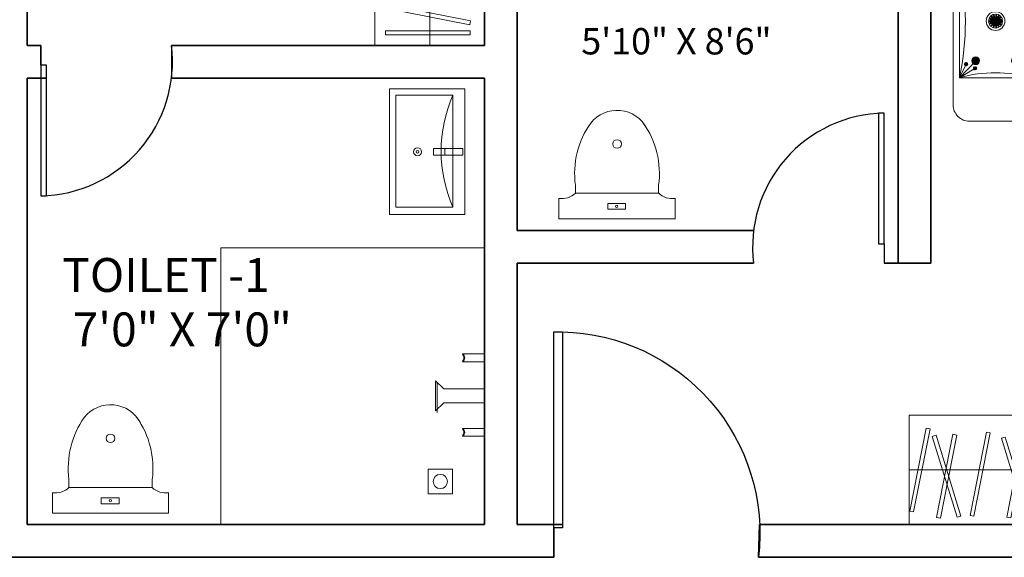
# Model space of a CAD drawing. Units: inches. Extents: x -61 to 1599, y -1316 to 257.
# Tile 171 of 204: x 1214 to 1395, y -783 to -684. Entities that reach past the tile are written whole.
import ezdxf

# ---------------------------------------------------------------- set-up
doc = ezdxf.new("R2010")
doc.units = ezdxf.units.IN
doc.header["$MEASUREMENT"] = 0
doc.linetypes.add('ACAD_ISO02W100', pattern=[15, 12, -3])
for name, color, linetype, lineweight in [('A-AREA-IDEN', 1, 'Continuous', 18), ('A-FLOR-CASE', 8, 'Continuous', 18), ('A-FLOR-FIXT', 8, 'Continuous', 18), ('A-WALL-JAMB', 4, 'ACAD_ISO02W100', 25), ('DOORS', 2, 'Continuous', 25), ('FURNITURE', 83, 'Continuous', 18), ('WALLS', 4, 'Continuous', 35)]:
    doc.layers.add(name, color=color, linetype=linetype, lineweight=lineweight)
doc.layers.add('LT', color=8, linetype='Continuous')
doc.styles.get("Standard").update_dxf_attribs({"font": 'arial.ttf'})

# ---------------------------------------------------------------- blocks, each defined once
blk = doc.blocks.new('DOOR-SWING-24')
blk.add_line((0, 0), (0, 3.6))
blk.add_lwpolyline([(0, 0), (0, -24), (1.05, -24), (1.05, 0)], close=True)
blk.add_arc((-0.44, 0.62), 24.62, 271.0259, 6.9559)
blk = doc.blocks.new('DOOR-SWING-36')
blk.add_line((0, 0), (0, -5.4))
blk.add_lwpolyline([(0, 0), (0, 36), (-1.57, 36), (-1.57, 0)], close=True)
blk.add_arc((-0.74, -1.08), 37.09, 91.2913, 186.6905)
blk = doc.blocks.new('WC-FLOOR-MOUNT')
for p, q in [((3.02, 4.69), (3.02, 6.17)), ((18.31, 4.69), (18.31, 6.17)), ((0, 0), (0, 3.75)), ((3.02, 4.69), (18.31, 4.69)), ((21.33, 0), (21.33, 3.75)), ((0, 0), (21.33, 0))]:
    blk.add_line(p, q)
blk.add_lwpolyline([(12.24, 1.73), (8.96, 1.73), (8.96, 2.81), (12.24, 2.81)], close=True)
for centre, radius in [((10.67, 13.73), 0.792), ((10.6, 2.27), 0.208)]:
    blk.add_circle(centre, radius)
for centre, radius, start, end in [((10.67, 13.73), 6.18, 27.6844, 141.4697), ((19.05, 8.26), 16.17, 144.824, 187.4232), ((2.28, 8.26), 16.17, 352.5768, 35.176), ((0.56, 7.25), 3.55, 260.8586, 313.6993), ((20.77, 7.25), 3.55, 226.3007, 279.1414)]:
    blk.add_arc(centre, radius, start, end)
blk = doc.blocks.new('LAVATORY-WALL')
blk.add_line((10.19, 12.11), (10.19, 10.88))
for points in [[(13.87, 0), (0, 0), (0, 23.07), (13.87, 23.07)], [(13.87, 0), (0, 0), (0, 23.07), (13.87, 23.07)], [(1.2, 1.34), (1.2, 21.88), (11.67, 21.88), (11.67, 1.34)], [(8.09, 10.88), (8.09, 12.11), (13.47, 12.11), (13.47, 10.88)]]:
    blk.add_lwpolyline(points, close=True)
for radius in [0.74, 0.233]:
    blk.add_circle((5.16, 11.5), radius)
blk.add_arc((34.73, 11.61), 25.25, 155.9939, 204.0061)
blk = doc.blocks.new('SHOWER-FITTINGS')
for p, q in [((10.35, 25.72), (6.31, 25.72)), ((10.35, 24.3), (6.31, 24.3)), ((10.35, 23), (10.35, 23)), ((2.92, 19.29), (1.4, 20.76)), ((1.4, 15.27), (1.4, 20.76)), ((1.69, 14.98), (1.69, 20.48)), ((10.35, 19.29), (2.92, 19.29)), ((2.92, 16.74), (1.4, 15.27)), ((10.35, 16.74), (2.92, 16.74)), ((10.35, 12.03), (6.31, 12.03)), ((10.35, 10.61), (6.31, 10.61))]:
    blk.add_line(p, q)
blk.add_lwpolyline([(4.52, 0), (0, 0), (0, 4.57), (4.52, 4.57)], close=True)
blk.add_circle((2.26, 2.29), 1.31)
for points in [[(6.31, 24.3), (6.45, 24.53), (6.75, 25), (6.46, 25.48), (6.31, 25.72)], [(6.45, 24.3), (6.59, 24.53), (6.88, 25), (6.59, 25.48), (6.45, 25.72)], [(6.31, 10.61), (6.45, 10.84), (6.75, 11.31), (6.46, 11.78), (6.31, 12.03)], [(6.45, 10.61), (6.59, 10.84), (6.88, 11.31), (6.59, 11.78), (6.45, 12.03)]]:
    blk.add_open_spline(points, degree=3, knots=[0, 0, 0, 0, 0.7501, 1.532449, 1.532449, 1.532449, 1.532449])
blk = doc.blocks.new('WARDROBE-HANGING')
blk.add_line((10.05, 0), (10.05, 68))
for points in [[(20.09, 0), (0, 0), (0, 68), (20.09, 68)], [(2.48, 67.85), (17.75, 64.85), (17.61, 64.14), (2.34, 67.15)], [(1.35, 59.16), (16.22, 63.73), (16.43, 63.04), (1.56, 58.47)], [(1.32, 62.96), (16.59, 59.95), (16.45, 59.25), (1.19, 62.25)], [(1.71, 56.78), (16.98, 53.78), (16.84, 53.07), (1.57, 56.08)], [(1, 46.47), (15.87, 51.04), (16.08, 50.35), (1.21, 45.78)], [(1.39, 50.01), (16.66, 47.01), (16.52, 46.3), (1.26, 49.31)], [(1.36, 44.09), (16.63, 41.09), (16.49, 40.38), (1.23, 43.38)], [(1.26, 37.2), (16.53, 34.2), (16.39, 33.49), (1.12, 36.5)], [(1.28, 33.41), (16.16, 37.98), (16.37, 37.29), (1.49, 32.72)], [(1.65, 31.03), (16.92, 28.03), (16.78, 27.32), (1.51, 30.32)], [(1.28, 21.3), (16.15, 25.87), (16.36, 25.18), (1.49, 20.61)], [(1.26, 25.09), (16.53, 22.09), (16.39, 21.38), (1.12, 24.39)], [(1.65, 18.92), (16.91, 15.92), (16.78, 15.21), (1.51, 18.21)], [(1.91, 13.69), (17.17, 10.68), (17.04, 9.98), (1.77, 12.98)], [(1.93, 9.89), (16.8, 14.46), (17.01, 13.77), (2.14, 9.2)], [(2.29, 7.51), (17.56, 4.51), (17.42, 3.8), (2.16, 6.81)], [(17.49, 1.96), (1.93, 1.96), (1.93, 2.68), (17.49, 2.68)]]:
    blk.add_lwpolyline(points, close=True)
blk = doc.blocks.new('*U100')
at = {"layer": 'LT'}
blk.add_line((0, 0.15), (0, -0.15), dxfattribs=at)
for centre, start, end in [((0.44, 0), 160.9983, 199.0017), ((-0.44, 0), 340.9983, 19.0017)]:
    blk.add_arc(centre, 0.468, start, end, dxfattribs=at)
blk = doc.blocks.new('*U101')
at = {"layer": 'LT', "transparency": 16777216}
for p, rotation in [((-57.96, -16.31), 72), ((-57.93, -16.26), 48.00000000000001), ((-57.87, -16.22), 24), ((-57.75, -16.22), 336), ((-57.7, -16.26), 312), ((-57.67, -16.31), 288), ((-57.96, -16.37), 96), ((-57.94, -16.43), 120), ((-57.9, -16.48), 144), ((-57.84, -16.51), 168.0000000000001), ((-57.78, -16.51), 192), ((-57.72, -16.48), 216), ((-57.68, -16.43), 240), ((-57.66, -16.37), 264)]:
    blk.add_blockref('*U100', p, dxfattribs=dict(at, rotation=rotation))
blk.add_blockref('*U100', (-57.81, -16.21), dxfattribs=at)
blk = doc.blocks.new('*U104')
at = {"layer": 'LT'}
blk.add_line((0, 0.15), (0, -0.15), dxfattribs=at)
for centre, start, end in [((0.44, 0), 160.9983, 199.0017), ((-0.44, 0), 340.9983, 19.0017)]:
    blk.add_arc(centre, 0.468, start, end, dxfattribs=at)
blk = doc.blocks.new('*U105')
at = {"layer": 'LT', "transparency": 16777216}
for p, rotation in [((-57.96, -16.31), 72), ((-57.93, -16.26), 48.00000000000001), ((-57.87, -16.22), 24), ((-57.75, -16.22), 336), ((-57.7, -16.26), 312), ((-57.67, -16.31), 288), ((-57.96, -16.37), 96), ((-57.94, -16.43), 120), ((-57.9, -16.48), 144), ((-57.84, -16.51), 168.0000000000001), ((-57.78, -16.51), 192), ((-57.72, -16.48), 216), ((-57.68, -16.43), 240), ((-57.66, -16.37), 264)]:
    blk.add_blockref('*U104', p, dxfattribs=dict(at, rotation=rotation))
blk.add_blockref('*U104', (-57.81, -16.21), dxfattribs=at)
blk = doc.blocks.new('*U71')
at = {"layer": 'LT'}
blk.add_line((0, 0.15), (0, -0.15), dxfattribs=at)
for centre, start, end in [((0.44, 0), 160.9983, 199.0017), ((-0.44, 0), 340.9983, 19.0017)]:
    blk.add_arc(centre, 0.468, start, end, dxfattribs=at)
blk = doc.blocks.new('*U58')
at = {"layer": 'LT', "transparency": 16777216}
for p, rotation in [((-57.96, -16.31), 72), ((-57.93, -16.26), 48.00000000000001), ((-57.87, -16.22), 24), ((-57.75, -16.22), 336), ((-57.7, -16.26), 312), ((-57.67, -16.31), 288), ((-57.96, -16.37), 96), ((-57.94, -16.43), 120), ((-57.9, -16.48), 144), ((-57.84, -16.51), 168.0000000000001), ((-57.78, -16.51), 192), ((-57.72, -16.48), 216), ((-57.68, -16.43), 240), ((-57.66, -16.37), 264)]:
    blk.add_blockref('*U71', p, dxfattribs=dict(at, rotation=rotation))
blk.add_blockref('*U71', (-57.81, -16.21), dxfattribs=at)
blk = doc.blocks.new('*U61')
at = {"layer": 'LT'}
blk.add_line((0, 0.15), (0, -0.15), dxfattribs=at)
for centre, start, end in [((0.44, 0), 160.9983, 199.0017), ((-0.44, 0), 340.9983, 19.0017)]:
    blk.add_arc(centre, 0.468, start, end, dxfattribs=at)
blk = doc.blocks.new('*U62')
at = {"layer": 'LT', "transparency": 16777216}
for p, rotation in [((-57.96, -16.31), 72), ((-57.93, -16.26), 48.00000000000001), ((-57.87, -16.22), 24), ((-57.75, -16.22), 336), ((-57.7, -16.26), 312), ((-57.67, -16.31), 288), ((-57.96, -16.37), 96), ((-57.94, -16.43), 120), ((-57.9, -16.48), 144), ((-57.84, -16.51), 168.0000000000001), ((-57.78, -16.51), 192), ((-57.72, -16.48), 216), ((-57.68, -16.43), 240), ((-57.66, -16.37), 264)]:
    blk.add_blockref('*U61', p, dxfattribs=dict(at, rotation=rotation))
blk.add_blockref('*U61', (-57.81, -16.21), dxfattribs=at)
blk = doc.blocks.new('*U94')
at = {"layer": 'LT'}
blk.add_line((0, 0.36), (0, -0.36), dxfattribs=at)
for centre, start, end in [((1.04, 0), 160.9983, 199.0017), ((-1.04, 0), 340.9983, 19.0017)]:
    blk.add_arc(centre, 1.1, start, end, dxfattribs=at)
blk = doc.blocks.new('*U95')
at = {"layer": 'LT', "transparency": 16777216}
for p, rotation in [((-136.23, -38.23), 48.00000000000001), ((-136.11, -38.14), 23.99999999999999), ((-135.82, -38.14), 336.0000000000001), ((-135.69, -38.23), 312), ((-136.32, -38.51), 96), ((-136.3, -38.36), 72), ((-136.27, -38.65), 120), ((-136.17, -38.76), 144), ((-136.04, -38.82), 168.0000000000001), ((-135.89, -38.82), 191.9999999999999), ((-135.75, -38.76), 216), ((-135.65, -38.65), 240), ((-135.62, -38.36), 288.0000000000001), ((-135.6, -38.51), 264)]:
    blk.add_blockref('*U94', p, dxfattribs=dict(at, rotation=rotation))
blk.add_blockref('*U94', (-135.96, -38.11), dxfattribs=at)
blk = doc.blocks.new('*U57')
at = {"layer": 'LT'}
blk.add_line((0, 0.36), (0, -0.36), dxfattribs=at)
for centre, start, end in [((1.04, 0), 160.9983, 199.0017), ((-1.04, 0), 340.9983, 19.0017)]:
    blk.add_arc(centre, 1.1, start, end, dxfattribs=at)
blk = doc.blocks.new('*U99')
at = {"layer": 'LT', "transparency": 16777216}
for p, rotation in [((-136.23, -38.23), 48.00000000000001), ((-136.11, -38.14), 23.99999999999999), ((-135.82, -38.14), 336.0000000000001), ((-135.69, -38.23), 312), ((-136.32, -38.51), 96), ((-136.3, -38.36), 72), ((-136.27, -38.65), 120), ((-136.17, -38.76), 144), ((-136.04, -38.82), 168.0000000000001), ((-135.89, -38.82), 191.9999999999999), ((-135.75, -38.76), 216), ((-135.65, -38.65), 240), ((-135.62, -38.36), 288.0000000000001), ((-135.6, -38.51), 264)]:
    blk.add_blockref('*U57', p, dxfattribs=dict(at, rotation=rotation))
blk.add_blockref('*U57', (-135.96, -38.11), dxfattribs=at)
blk = doc.blocks.new('*U80')
at = {"layer": 'LT'}
blk.add_line((0, 0.36), (0, -0.36), dxfattribs=at)
for centre, start, end in [((1.04, 0), 160.9983, 199.0017), ((-1.04, 0), 340.9983, 19.0017)]:
    blk.add_arc(centre, 1.1, start, end, dxfattribs=at)
blk = doc.blocks.new('*U96')
at = {"layer": 'LT', "transparency": 16777216}
for p, rotation in [((-136.23, -38.23), 48.00000000000001), ((-136.11, -38.14), 23.99999999999999), ((-135.82, -38.14), 336.0000000000001), ((-135.69, -38.23), 312), ((-136.32, -38.51), 96), ((-136.3, -38.36), 72), ((-136.27, -38.65), 120), ((-136.17, -38.76), 144), ((-136.04, -38.82), 168.0000000000001), ((-135.89, -38.82), 191.9999999999999), ((-135.75, -38.76), 216), ((-135.65, -38.65), 240), ((-135.62, -38.36), 288.0000000000001), ((-135.6, -38.51), 264)]:
    blk.add_blockref('*U80', p, dxfattribs=dict(at, rotation=rotation))
blk.add_blockref('*U80', (-135.96, -38.11), dxfattribs=at)
blk = doc.blocks.new('*U69')
at = {"layer": 'LT'}
blk.add_line((0, 0.36), (0, -0.36), dxfattribs=at)
for centre, start, end in [((1.04, 0), 160.9983, 199.0017), ((-1.04, 0), 340.9983, 19.0017)]:
    blk.add_arc(centre, 1.1, start, end, dxfattribs=at)
blk = doc.blocks.new('*U70')
at = {"layer": 'LT', "transparency": 16777216}
for p, rotation in [((-136.23, -38.23), 48.00000000000001), ((-136.11, -38.14), 23.99999999999999), ((-135.82, -38.14), 336.0000000000001), ((-135.69, -38.23), 312), ((-136.32, -38.51), 96), ((-136.3, -38.36), 72), ((-136.27, -38.65), 120), ((-136.17, -38.76), 144), ((-136.04, -38.82), 168.0000000000001), ((-135.89, -38.82), 191.9999999999999), ((-135.75, -38.76), 216), ((-135.65, -38.65), 240), ((-135.62, -38.36), 288.0000000000001), ((-135.6, -38.51), 264)]:
    blk.add_blockref('*U69', p, dxfattribs=dict(at, rotation=rotation))
blk.add_blockref('*U69', (-135.96, -38.11), dxfattribs=at)
blk = doc.blocks.new('*U102')
at = {"layer": 'LT'}
blk.add_line((0, 0.15), (0, -0.15), dxfattribs=at)
for centre, start, end in [((0.44, 0), 160.9983, 199.0017), ((-0.44, 0), 340.9983, 19.0017)]:
    blk.add_arc(centre, 0.468, start, end, dxfattribs=at)
blk = doc.blocks.new('*U103')
at = {"layer": 'LT', "transparency": 16777216}
for p, rotation in [((-57.96, -16.31), 72), ((-57.93, -16.26), 48.00000000000001), ((-57.87, -16.22), 24), ((-57.75, -16.22), 336), ((-57.7, -16.26), 312), ((-57.67, -16.31), 288), ((-57.96, -16.37), 96), ((-57.94, -16.43), 120), ((-57.9, -16.48), 144), ((-57.84, -16.51), 168.0000000000001), ((-57.78, -16.51), 192), ((-57.72, -16.48), 216), ((-57.68, -16.43), 240), ((-57.66, -16.37), 264)]:
    blk.add_blockref('*U102', p, dxfattribs=dict(at, rotation=rotation))
blk.add_blockref('*U102', (-57.81, -16.21), dxfattribs=at)
blk = doc.blocks.new('*U55')
at = {"layer": 'LT'}
blk.add_line((0, 0.15), (0, -0.15), dxfattribs=at)
for centre, start, end in [((0.44, 0), 160.9983, 199.0017), ((-0.44, 0), 340.9983, 19.0017)]:
    blk.add_arc(centre, 0.468, start, end, dxfattribs=at)
blk = doc.blocks.new('*U56')
at = {"layer": 'LT', "transparency": 16777216}
for p, rotation in [((-57.96, -16.31), 72), ((-57.93, -16.26), 48.00000000000001), ((-57.87, -16.22), 24), ((-57.75, -16.22), 336), ((-57.7, -16.26), 312), ((-57.67, -16.31), 288), ((-57.96, -16.37), 96), ((-57.94, -16.43), 120), ((-57.9, -16.48), 144), ((-57.84, -16.51), 168.0000000000001), ((-57.78, -16.51), 192), ((-57.72, -16.48), 216), ((-57.68, -16.43), 240), ((-57.66, -16.37), 264)]:
    blk.add_blockref('*U55', p, dxfattribs=dict(at, rotation=rotation))
blk.add_blockref('*U55', (-57.81, -16.21), dxfattribs=at)
blk = doc.blocks.new('*U59')
at = {"layer": 'LT'}
blk.add_line((0, 0.15), (0, -0.15), dxfattribs=at)
for centre, start, end in [((0.44, 0), 160.9983, 199.0017), ((-0.44, 0), 340.9983, 19.0017)]:
    blk.add_arc(centre, 0.468, start, end, dxfattribs=at)
blk = doc.blocks.new('*U60')
at = {"layer": 'LT', "transparency": 16777216}
for p, rotation in [((-57.96, -16.31), 72), ((-57.93, -16.26), 48.00000000000001), ((-57.87, -16.22), 24), ((-57.75, -16.22), 336), ((-57.7, -16.26), 312), ((-57.67, -16.31), 288), ((-57.96, -16.37), 96), ((-57.94, -16.43), 120), ((-57.9, -16.48), 144), ((-57.84, -16.51), 168.0000000000001), ((-57.78, -16.51), 192), ((-57.72, -16.48), 216), ((-57.68, -16.43), 240), ((-57.66, -16.37), 264)]:
    blk.add_blockref('*U59', p, dxfattribs=dict(at, rotation=rotation))
blk.add_blockref('*U59', (-57.81, -16.21), dxfattribs=at)
blk = doc.blocks.new('*U67')
at = {"layer": 'LT'}
blk.add_line((0, 0.15), (0, -0.15), dxfattribs=at)
for centre, start, end in [((0.44, 0), 160.9983, 199.0017), ((-0.44, 0), 340.9983, 19.0017)]:
    blk.add_arc(centre, 0.468, start, end, dxfattribs=at)
blk = doc.blocks.new('*U68')
at = {"layer": 'LT', "transparency": 16777216}
for p, rotation in [((-57.96, -16.31), 72), ((-57.93, -16.26), 48.00000000000001), ((-57.87, -16.22), 24), ((-57.75, -16.22), 336), ((-57.7, -16.26), 312), ((-57.67, -16.31), 288), ((-57.96, -16.37), 96), ((-57.94, -16.43), 120), ((-57.9, -16.48), 144), ((-57.84, -16.51), 168.0000000000001), ((-57.78, -16.51), 192), ((-57.72, -16.48), 216), ((-57.68, -16.43), 240), ((-57.66, -16.37), 264)]:
    blk.add_blockref('*U67', p, dxfattribs=dict(at, rotation=rotation))
blk.add_blockref('*U67', (-57.81, -16.21), dxfattribs=at)
blk = doc.blocks.new('*U106')
at = {"layer": 'LT'}
blk.add_line((0, 0.64), (0, -0.64), dxfattribs=at)
for centre, start, end in [((1.87, 0), 160.9983, 199.0017), ((-1.87, 0), 340.9983, 19.0017)]:
    blk.add_arc(centre, 1.97, start, end, dxfattribs=at)
blk = doc.blocks.new('*U93')
at = {"layer": 'LT', "transparency": 16777216}
for p, rotation in [((-244.33, -68.76), 72), ((-244.2, -68.53), 48.00000000000001), ((-243.98, -68.38), 23.99999999999999), ((-243.46, -68.38), 336.0000000000001), ((-243.25, -68.53), 312), ((-243.11, -68.76), 288), ((-244.36, -69.03), 96), ((-244.28, -69.28), 120), ((-244.1, -69.48), 144), ((-243.86, -69.59), 168), ((-243.59, -69.59), 192), ((-243.34, -69.48), 216), ((-243.17, -69.28), 240), ((-243.08, -69.03), 264)]:
    blk.add_blockref('*U106', p, dxfattribs=dict(at, rotation=rotation))
blk.add_blockref('*U106', (-243.72, -68.32), dxfattribs=at)
blk = doc.blocks.new('*U63')
at = {"layer": 'LT'}
blk.add_line((0, 0.64), (0, -0.64), dxfattribs=at)
for centre, start, end in [((1.87, 0), 160.9983, 199.0017), ((-1.87, 0), 340.9983, 19.0017)]:
    blk.add_arc(centre, 1.97, start, end, dxfattribs=at)
blk = doc.blocks.new('*U64')
at = {"layer": 'LT', "transparency": 16777216}
for p, rotation in [((-244.33, -68.76), 72), ((-244.2, -68.53), 48.00000000000001), ((-243.98, -68.38), 23.99999999999999), ((-243.46, -68.38), 336.0000000000001), ((-243.25, -68.53), 312), ((-243.11, -68.76), 288), ((-244.36, -69.03), 96), ((-244.28, -69.28), 120), ((-244.1, -69.48), 144), ((-243.86, -69.59), 168), ((-243.59, -69.59), 192), ((-243.34, -69.48), 216), ((-243.17, -69.28), 240), ((-243.08, -69.03), 264)]:
    blk.add_blockref('*U63', p, dxfattribs=dict(at, rotation=rotation))
blk.add_blockref('*U63', (-243.72, -68.32), dxfattribs=at)
blk = doc.blocks.new('*U83')
at = {"layer": 'LT'}
blk.add_line((0, 0.36), (0, -0.36), dxfattribs=at)
for centre, start, end in [((1.04, 0), 160.9983, 199.0017), ((-1.04, 0), 340.9983, 19.0017)]:
    blk.add_arc(centre, 1.1, start, end, dxfattribs=at)
blk = doc.blocks.new('*U84')
at = {"layer": 'LT', "transparency": 16777216}
for p, rotation in [((-136.23, -38.23), 48.00000000000001), ((-136.11, -38.14), 23.99999999999999), ((-135.82, -38.14), 336.0000000000001), ((-135.69, -38.23), 312), ((-136.32, -38.51), 96), ((-136.3, -38.36), 72), ((-136.27, -38.65), 120), ((-136.17, -38.76), 144), ((-136.04, -38.82), 168.0000000000001), ((-135.89, -38.82), 191.9999999999999), ((-135.75, -38.76), 216), ((-135.65, -38.65), 240), ((-135.62, -38.36), 288.0000000000001), ((-135.6, -38.51), 264)]:
    blk.add_blockref('*U83', p, dxfattribs=dict(at, rotation=rotation))
blk.add_blockref('*U83', (-135.96, -38.11), dxfattribs=at)
blk = doc.blocks.new('*U74')
at = {"layer": 'LT'}
blk.add_line((0, 0.36), (0, -0.36), dxfattribs=at)
for centre, start, end in [((1.04, 0), 160.9983, 199.0017), ((-1.04, 0), 340.9983, 19.0017)]:
    blk.add_arc(centre, 1.1, start, end, dxfattribs=at)
blk = doc.blocks.new('*U75')
at = {"layer": 'LT', "transparency": 16777216}
for p, rotation in [((-136.23, -38.23), 48.00000000000001), ((-136.11, -38.14), 23.99999999999999), ((-135.82, -38.14), 336.0000000000001), ((-135.69, -38.23), 312), ((-136.32, -38.51), 96), ((-136.3, -38.36), 72), ((-136.27, -38.65), 120), ((-136.17, -38.76), 144), ((-136.04, -38.82), 168.0000000000001), ((-135.89, -38.82), 191.9999999999999), ((-135.75, -38.76), 216), ((-135.65, -38.65), 240), ((-135.62, -38.36), 288.0000000000001), ((-135.6, -38.51), 264)]:
    blk.add_blockref('*U74', p, dxfattribs=dict(at, rotation=rotation))
blk.add_blockref('*U74', (-135.96, -38.11), dxfattribs=at)
blk = doc.blocks.new('*U65')
at = {"layer": 'LT'}
blk.add_line((0, 0.36), (0, -0.36), dxfattribs=at)
for centre, start, end in [((1.04, 0), 160.9983, 199.0017), ((-1.04, 0), 340.9983, 19.0017)]:
    blk.add_arc(centre, 1.1, start, end, dxfattribs=at)
blk = doc.blocks.new('*U66')
at = {"layer": 'LT', "transparency": 16777216}
for p, rotation in [((-136.23, -38.23), 48.00000000000001), ((-136.11, -38.14), 23.99999999999999), ((-135.82, -38.14), 336.0000000000001), ((-135.69, -38.23), 312), ((-136.32, -38.51), 96), ((-136.3, -38.36), 72), ((-136.27, -38.65), 120), ((-136.17, -38.76), 144), ((-136.04, -38.82), 168.0000000000001), ((-135.89, -38.82), 191.9999999999999), ((-135.75, -38.76), 216), ((-135.65, -38.65), 240), ((-135.62, -38.36), 288.0000000000001), ((-135.6, -38.51), 264)]:
    blk.add_blockref('*U65', p, dxfattribs=dict(at, rotation=rotation))
blk.add_blockref('*U65', (-135.96, -38.11), dxfattribs=at)
blk = doc.blocks.new('*U85')
at = {"layer": 'LT'}
blk.add_line((0, 0.36), (0, -0.36), dxfattribs=at)
for centre, start, end in [((1.04, 0), 160.9983, 199.0017), ((-1.04, 0), 340.9983, 19.0017)]:
    blk.add_arc(centre, 1.1, start, end, dxfattribs=at)
blk = doc.blocks.new('*U86')
at = {"layer": 'LT', "transparency": 16777216}
for p, rotation in [((-136.23, -38.23), 48.00000000000001), ((-136.11, -38.14), 23.99999999999999), ((-135.82, -38.14), 336.0000000000001), ((-135.69, -38.23), 312), ((-136.32, -38.51), 96), ((-136.3, -38.36), 72), ((-136.27, -38.65), 120), ((-136.17, -38.76), 144), ((-136.04, -38.82), 168.0000000000001), ((-135.89, -38.82), 191.9999999999999), ((-135.75, -38.76), 216), ((-135.65, -38.65), 240), ((-135.62, -38.36), 288.0000000000001), ((-135.6, -38.51), 264)]:
    blk.add_blockref('*U85', p, dxfattribs=dict(at, rotation=rotation))
blk.add_blockref('*U85', (-135.96, -38.11), dxfattribs=at)
blk = doc.blocks.new('*U78')
at = {"layer": 'LT'}
blk.add_line((0, 0.15), (0, -0.15), dxfattribs=at)
for centre, start, end in [((0.44, 0), 160.9983, 199.0017), ((-0.44, 0), 340.9983, 19.0017)]:
    blk.add_arc(centre, 0.468, start, end, dxfattribs=at)
blk = doc.blocks.new('*U79')
at = {"layer": 'LT', "transparency": 16777216}
for p, rotation in [((-57.96, -16.31), 72), ((-57.93, -16.26), 48.00000000000001), ((-57.87, -16.22), 24), ((-57.75, -16.22), 336), ((-57.7, -16.26), 312), ((-57.67, -16.31), 288), ((-57.96, -16.37), 96), ((-57.94, -16.43), 120), ((-57.9, -16.48), 144), ((-57.84, -16.51), 168.0000000000001), ((-57.78, -16.51), 192), ((-57.72, -16.48), 216), ((-57.68, -16.43), 240), ((-57.66, -16.37), 264)]:
    blk.add_blockref('*U78', p, dxfattribs=dict(at, rotation=rotation))
blk.add_blockref('*U78', (-57.81, -16.21), dxfattribs=at)
blk = doc.blocks.new('*U72')
at = {"layer": 'LT'}
blk.add_line((0, 0.15), (0, -0.15), dxfattribs=at)
for centre, start, end in [((0.44, 0), 160.9983, 199.0017), ((-0.44, 0), 340.9983, 19.0017)]:
    blk.add_arc(centre, 0.468, start, end, dxfattribs=at)
blk = doc.blocks.new('*U73')
at = {"layer": 'LT', "transparency": 16777216}
for p, rotation in [((-57.96, -16.31), 72), ((-57.93, -16.26), 48.00000000000001), ((-57.87, -16.22), 24), ((-57.75, -16.22), 336), ((-57.7, -16.26), 312), ((-57.67, -16.31), 288), ((-57.96, -16.37), 96), ((-57.94, -16.43), 120), ((-57.9, -16.48), 144), ((-57.84, -16.51), 168.0000000000001), ((-57.78, -16.51), 192), ((-57.72, -16.48), 216), ((-57.68, -16.43), 240), ((-57.66, -16.37), 264)]:
    blk.add_blockref('*U72', p, dxfattribs=dict(at, rotation=rotation))
blk.add_blockref('*U72', (-57.81, -16.21), dxfattribs=at)
blk = doc.blocks.new('*U89')
at = {"layer": 'LT'}
blk.add_line((0, 0.15), (0, -0.15), dxfattribs=at)
for centre, start, end in [((0.44, 0), 160.9983, 199.0017), ((-0.44, 0), 340.9983, 19.0017)]:
    blk.add_arc(centre, 0.468, start, end, dxfattribs=at)
blk = doc.blocks.new('*U90')
at = {"layer": 'LT', "transparency": 16777216}
for p, rotation in [((-57.96, -16.31), 72), ((-57.93, -16.26), 48.00000000000001), ((-57.87, -16.22), 24), ((-57.75, -16.22), 336), ((-57.7, -16.26), 312), ((-57.67, -16.31), 288), ((-57.96, -16.37), 96), ((-57.94, -16.43), 120), ((-57.9, -16.48), 144), ((-57.84, -16.51), 168.0000000000001), ((-57.78, -16.51), 192), ((-57.72, -16.48), 216), ((-57.68, -16.43), 240), ((-57.66, -16.37), 264)]:
    blk.add_blockref('*U89', p, dxfattribs=dict(at, rotation=rotation))
blk.add_blockref('*U89', (-57.81, -16.21), dxfattribs=at)
blk = doc.blocks.new('*U97')
at = {"layer": 'LT'}
blk.add_line((0, 0.15), (0, -0.15), dxfattribs=at)
for centre, start, end in [((0.44, 0), 160.9983, 199.0017), ((-0.44, 0), 340.9983, 19.0017)]:
    blk.add_arc(centre, 0.468, start, end, dxfattribs=at)
blk = doc.blocks.new('*U98')
at = {"layer": 'LT', "transparency": 16777216}
for p, rotation in [((-57.96, -16.31), 72), ((-57.93, -16.26), 48.00000000000001), ((-57.87, -16.22), 24), ((-57.75, -16.22), 336), ((-57.7, -16.26), 312), ((-57.67, -16.31), 288), ((-57.96, -16.37), 96), ((-57.94, -16.43), 120), ((-57.9, -16.48), 144), ((-57.84, -16.51), 168.0000000000001), ((-57.78, -16.51), 192), ((-57.72, -16.48), 216), ((-57.68, -16.43), 240), ((-57.66, -16.37), 264)]:
    blk.add_blockref('*U97', p, dxfattribs=dict(at, rotation=rotation))
blk.add_blockref('*U97', (-57.81, -16.21), dxfattribs=at)
blk = doc.blocks.new('*U76')
at = {"layer": 'LT'}
blk.add_line((0, 0.15), (0, -0.15), dxfattribs=at)
for centre, start, end in [((0.44, 0), 160.9983, 199.0017), ((-0.44, 0), 340.9983, 19.0017)]:
    blk.add_arc(centre, 0.468, start, end, dxfattribs=at)
blk = doc.blocks.new('*U77')
at = {"layer": 'LT', "transparency": 16777216}
for p, rotation in [((-57.96, -16.31), 72), ((-57.93, -16.26), 48.00000000000001), ((-57.87, -16.22), 24), ((-57.75, -16.22), 336), ((-57.7, -16.26), 312), ((-57.67, -16.31), 288), ((-57.96, -16.37), 96), ((-57.94, -16.43), 120), ((-57.9, -16.48), 144), ((-57.84, -16.51), 168.0000000000001), ((-57.78, -16.51), 192), ((-57.72, -16.48), 216), ((-57.68, -16.43), 240), ((-57.66, -16.37), 264)]:
    blk.add_blockref('*U76', p, dxfattribs=dict(at, rotation=rotation))
blk.add_blockref('*U76', (-57.81, -16.21), dxfattribs=at)
blk = doc.blocks.new('*U81')
at = {"layer": 'LT'}
blk.add_line((0, 0.15), (0, -0.15), dxfattribs=at)
for centre, start, end in [((0.44, 0), 160.9983, 199.0017), ((-0.44, 0), 340.9983, 19.0017)]:
    blk.add_arc(centre, 0.468, start, end, dxfattribs=at)
blk = doc.blocks.new('*U82')
at = {"layer": 'LT', "transparency": 16777216}
for p, rotation in [((-57.96, -16.31), 72), ((-57.93, -16.26), 48.00000000000001), ((-57.87, -16.22), 24), ((-57.75, -16.22), 336), ((-57.7, -16.26), 312), ((-57.67, -16.31), 288), ((-57.96, -16.37), 96), ((-57.94, -16.43), 120), ((-57.9, -16.48), 144), ((-57.84, -16.51), 168.0000000000001), ((-57.78, -16.51), 192), ((-57.72, -16.48), 216), ((-57.68, -16.43), 240), ((-57.66, -16.37), 264)]:
    blk.add_blockref('*U81', p, dxfattribs=dict(at, rotation=rotation))
blk.add_blockref('*U81', (-57.81, -16.21), dxfattribs=at)
blk = doc.blocks.new('*U87')
at = {"layer": 'LT'}
blk.add_line((0, 0.15), (0, -0.15), dxfattribs=at)
for centre, start, end in [((0.44, 0), 160.9983, 199.0017), ((-0.44, 0), 340.9983, 19.0017)]:
    blk.add_arc(centre, 0.468, start, end, dxfattribs=at)
blk = doc.blocks.new('*U88')
at = {"layer": 'LT', "transparency": 16777216}
for p, rotation in [((-57.96, -16.31), 72), ((-57.93, -16.26), 48.00000000000001), ((-57.87, -16.22), 24), ((-57.75, -16.22), 336), ((-57.7, -16.26), 312), ((-57.67, -16.31), 288), ((-57.96, -16.37), 96), ((-57.94, -16.43), 120), ((-57.9, -16.48), 144), ((-57.84, -16.51), 168.0000000000001), ((-57.78, -16.51), 192), ((-57.72, -16.48), 216), ((-57.68, -16.43), 240), ((-57.66, -16.37), 264)]:
    blk.add_blockref('*U87', p, dxfattribs=dict(at, rotation=rotation))
blk.add_blockref('*U87', (-57.81, -16.21), dxfattribs=at)
blk = doc.blocks.new('*U91')
at = {"layer": 'LT'}
blk.add_line((0, 0.15), (0, -0.15), dxfattribs=at)
for centre, start, end in [((0.44, 0), 160.9983, 199.0017), ((-0.44, 0), 340.9983, 19.0017)]:
    blk.add_arc(centre, 0.468, start, end, dxfattribs=at)
blk = doc.blocks.new('*U92')
at = {"layer": 'LT', "transparency": 16777216}
for p, rotation in [((-57.96, -16.31), 72), ((-57.93, -16.26), 48.00000000000001), ((-57.87, -16.22), 24), ((-57.75, -16.22), 336), ((-57.7, -16.26), 312), ((-57.67, -16.31), 288), ((-57.96, -16.37), 96), ((-57.94, -16.43), 120), ((-57.9, -16.48), 144), ((-57.84, -16.51), 168.0000000000001), ((-57.78, -16.51), 192), ((-57.72, -16.48), 216), ((-57.68, -16.43), 240), ((-57.66, -16.37), 264)]:
    blk.add_blockref('*U91', p, dxfattribs=dict(at, rotation=rotation))
blk.add_blockref('*U91', (-57.81, -16.21), dxfattribs=at)
blk = doc.blocks.new('BED-DOUBLE-COMPACT')
for p, q in [((16.8, 60.04), (16.8, 0.04)), ((17.8, 60.04), (17.8, 0.04)), ((1.2, 52.04), (14.4, 52.04)), ((1.2, 52.04), (2.4, 49.53)), ((1.2, 52.04), (4.2, 48.93)), ((1.2, 52.04), (4.03, 50.31)), ((14.4, 52.04), (11.4, 48.93)), ((14.4, 52.04), (11.57, 50.31)), ((14.4, 52.04), (13.2, 49.53)), ((14.4, 31.24), (14.4, 52.04)), ((2.4, 49.53), (2.7, 49.53)), ((4.03, 50.31), (4.33, 50.31)), ((4.16, 48.92), (4.88, 48.92)), ((11.44, 48.92), (10.72, 48.92)), ((11.57, 50.31), (11.27, 50.31)), ((13.2, 49.53), (12.9, 49.53)), ((7.8, 41.64), (9.09, 41.64)), ((1.2, 31.24), (4.2, 34.34)), ((1.2, 31.24), (2.4, 33.74)), ((1.2, 31.24), (4.03, 32.96)), ((2.4, 33.74), (2.7, 33.74)), ((4.03, 32.96), (4.33, 32.96)), ((4.16, 34.35), (4.88, 34.35)), ((11.44, 34.35), (10.72, 34.35)), ((11.57, 32.96), (11.27, 32.96)), ((14.4, 31.24), (11.4, 34.34)), ((14.4, 31.24), (11.57, 32.96)), ((13.2, 33.74), (12.9, 33.74)), ((14.4, 31.24), (13.2, 33.74)), ((1.2, 31.24), (1.2, 31.24)), ((1.2, 28.84), (14.4, 28.84)), ((1.2, 28.84), (2.4, 26.33)), ((1.2, 28.84), (4.2, 25.73)), ((1.2, 28.84), (4.03, 27.11)), ((14.4, 28.84), (11.4, 25.73)), ((14.4, 28.84), (11.57, 27.11)), ((14.4, 28.84), (13.2, 26.33)), ((14.4, 8.04), (14.4, 28.84)), ((2.4, 26.33), (2.7, 26.33)), ((4.03, 27.11), (4.33, 27.11)), ((4.16, 25.72), (4.88, 25.72)), ((11.44, 25.72), (10.72, 25.72)), ((11.57, 27.11), (11.27, 27.11)), ((13.2, 26.33), (12.9, 26.33)), ((7.8, 18.44), (9.09, 18.44)), ((1.2, 8.04), (4.2, 11.14)), ((4.16, 11.15), (4.88, 11.15)), ((11.44, 11.15), (10.72, 11.15)), ((14.4, 8.04), (11.4, 11.14)), ((1.2, 8.04), (2.4, 10.54)), ((1.2, 8.04), (4.03, 9.76)), ((2.4, 10.54), (2.7, 10.54)), ((4.03, 9.76), (4.33, 9.76)), ((11.57, 9.76), (11.27, 9.76)), ((14.4, 8.04), (11.57, 9.76)), ((13.2, 10.54), (12.9, 10.54)), ((14.4, 8.04), (13.2, 10.54)), ((1.2, 8.04), (1.2, 8.04))]:
    blk.add_line(p, q)
for points in [[(77, 60.04), (3, 60.04, 0.414214), (0, 57.04), (0, 3.04, 0.414214), (3, 0.04), (77, 0.04, 0.414214), (80, 3.04), (80, 57.04, 0.414214)], [(2.7, 49.53, 0.167358), (2.4, 49.53, 0.167358)], [(4.33, 50.31, 0.167358), (4.03, 50.31, 0.167358)], [(4.88, 48.92, 0.167358), (4.16, 48.92, 0.167358)], [(11.44, 48.92, 0.167358), (10.72, 48.92, 0.167358)], [(11.57, 50.31, 0.167358), (11.27, 50.31, 0.167358)], [(13.2, 49.53, 0.167358), (12.9, 49.53, 0.167358)], [(7.8, 41.64, 0.167358), (9.09, 41.64, 0.167358)], [(4.16, 34.35, 0.167358), (4.88, 34.35, 0.167358)], [(10.72, 34.35, 0.167358), (11.44, 34.35, 0.167358)], [(2.4, 33.74, 0.167358), (2.7, 33.74, 0.167358)], [(4.03, 32.96, 0.167358), (4.33, 32.96, 0.167358)], [(11.27, 32.96, 0.167358), (11.57, 32.96, 0.167358)], [(4.33, 27.11, 0.167358), (4.03, 27.11, 0.167358)], [(11.57, 27.11, 0.167358), (11.27, 27.11, 0.167358)], [(35.77, 28.09, 0.064396), (48.86, 1.19, 0.181766), (36.45, 0.6, -0.202767)], [(2.7, 26.33, 0.167358), (2.4, 26.33, 0.167358)], [(4.88, 25.72, 0.167358), (4.16, 25.72, 0.167358)], [(11.44, 25.72, 0.167358), (10.72, 25.72, 0.167358)], [(13.2, 26.33, 0.167358), (12.9, 26.33, 0.167358)], [(7.8, 18.44, 0.167358), (9.09, 18.44, 0.167358)], [(4.16, 11.15, 0.167358), (4.88, 11.15, 0.167358)], [(10.72, 11.15, 0.167358), (11.44, 11.15, 0.167358)], [(2.4, 10.54, 0.167358), (2.7, 10.54, 0.167358)], [(4.03, 9.76, 0.167358), (4.33, 9.76, 0.167358)], [(11.27, 9.76, 0.167358), (11.57, 9.76, 0.167358)]]:
    blk.add_lwpolyline(points, format="xyb", close=True)
blk.add_lwpolyline([(36, 0.04, -0.22309), (36, 30.04, 0.142156), (36, 60.04)], format="xyb")
for points in [[(14.4, 31.24), (1.2, 31.24), (1.2, 52.04), (14.4, 52.04), (14.4, 31.24), (1.2, 31.24), (1.2, 52.04)], [(14.4, 8.04), (1.2, 8.04), (1.2, 28.84)]]:
    blk.add_lwpolyline(points)
for centre, radius in [((2.4, 49.53), 0.305), ((4.16, 48.92), 0.717), ((4.03, 50.31), 0.305), ((11.44, 48.92), 0.717), ((11.57, 50.31), 0.305), ((13.2, 49.53), 0.305), ((7.8, 41.64), 1.72), ((7.8, 41.64), 1.29), ((4.16, 34.35), 0.717), ((11.44, 34.35), 0.717), ((2.4, 33.74), 0.305), ((4.03, 32.96), 0.305), ((11.57, 32.96), 0.305), ((13.2, 33.74), 0.305), ((4.03, 27.11), 0.305), ((11.57, 27.11), 0.305), ((2.4, 26.33), 0.305), ((4.16, 25.72), 0.717), ((11.44, 25.72), 0.717), ((13.2, 26.33), 0.305), ((7.8, 18.44), 1.72), ((7.8, 18.44), 1.29), ((4.16, 11.15), 0.717), ((11.44, 11.15), 0.717), ((2.4, 10.54), 0.305), ((4.03, 9.76), 0.305), ((11.57, 9.76), 0.305), ((13.2, 10.54), 0.305)]:
    blk.add_circle(centre, radius)
for centre, radius, start, end in [((-49.23, 41.64), 51.49, 348.3468, 11.6532), ((7.8, 75.06), 23.95, 254.0046, 285.9954), ((64.83, 41.64), 51.49, 168.3468, 191.6532), ((13.05, 33.3), 0.468, 70.9983, 109.0017), ((13.05, 34.18), 0.468, 250.9983, 289.0017), ((7.8, 8.21), 23.95, 74.0046, 105.9954), ((-49.23, 18.44), 51.49, 348.3468, 11.6532), ((7.8, 51.86), 23.95, 254.0046, 285.9954), ((64.83, 18.44), 51.49, 168.3468, 191.6532), ((13.05, 10.1), 0.468, 70.9983, 109.0017), ((13.05, 10.98), 0.468, 250.9983, 289.0017), ((7.8, -14.99), 23.95, 74.0046, 105.9954)]:
    blk.add_arc(centre, radius, start, end)
for points, weights, knots in [([(50.36, 0.04), (44.31, 9.08), (39.57, 18.88), (36.25, 29.24), (36.33, 29.43), (36.41, 29.62), (36.5, 29.81), (39.38, 39.75), (39.36, 50.11), (36.43, 60.04), (39.05, 58.77), (44.5, 56.15), (52.79, 61.02), (60.85, 55.2), (67.65, 61.05), (73.39, 57.36), (75.56, 56.45)], [1, 0.993520320424, 0.993520320424, 1, 0.99997444972, 0.99997444972, 1, 0.973174868659, 0.973174868659, 1, 1, 1, 1, 1, 1, 1, 1], [0, 0, 0, 0, 0.279074, 0.279074, 0.279074, 0.296584, 0.296584, 0.296584, 0.865868, 0.865868, 0.865868, 9.142578, 18.107734, 25.769226, 34.110801, 40.441511, 40.441511, 40.441511, 40.441511]), ([(36.38, 0.04), (40.9, 1.99), (45.83, 1.99), (50.36, 0.04), (52.47, 1.05), (56.42, 2.94), (63, -0.48), (69.27, 4.67), (73.92, -0.77), (76.3, 0.25), (77.18, 0.91)], [1, 0.945466318698, 0.945466318698, 1, 1, 1, 1, 1, 1, 1, 1], [0, 0, 0, 0, 0.814571, 0.814571, 0.814571, 7.464247, 13.266353, 20.788537, 26.138745, 29.321895, 29.321895, 29.321895, 29.321895])]:
    blk.add_rational_spline(points, weights, degree=3, knots=knots)
for points, knots in [([(78.07, 0.04), (75.8, 2.26), (70.92, 7.04), (82.19, 15.5), (70.03, 25.56), (82.2, 36.26), (68.97, 47.49), (74.96, 55.75), (78.07, 60.04)], [0, 0, 0, 0, 7.980285, 17.179806, 28.830278, 39.318084, 52.078264, 65.891546, 65.891546, 65.891546, 65.891546]), ([(80, 0.04), (77.73, 2.26), (72.85, 7.04), (84.12, 15.5), (71.96, 25.56), (84.13, 36.26), (70.9, 47.49), (76.89, 55.75), (80, 60.04)], [0, 0, 0, 0, 7.980285, 17.179806, 28.830278, 39.318084, 52.078264, 65.891546, 65.891546, 65.891546, 65.891546]), ([(36.91, 58.31), (39.53, 57.05), (44.98, 54.43), (53.27, 59.3), (61.33, 53.48), (67.78, 59.03), (72.97, 56.17), (74.83, 55.28)], [0, 0, 0, 0, 8.27671, 17.241866, 24.903358, 33.244933, 38.427294, 38.427294, 38.427294, 38.427294]), ([(49.89, 0.74), (52, 1.75), (55.95, 3.65), (62.54, 0.23), (68.8, 5.38), (73.4, -0.01), (75.74, 0.92), (76.58, 1.52)], [0, 0, 0, 0, 6.649676, 12.451782, 19.973966, 25.324174, 28.349676, 28.349676, 28.349676, 28.349676])]:
    blk.add_open_spline(points, degree=3, knots=knots)
blk.add_open_spline([(80, 56.78), (80.02, 56.81), (80.03, 56.83), (80.05, 56.85)], degree=3)
at = {"xscale": -1}
for name, p, rotation in [('*U62', (-13.96, -8.28), 90), ('*U70', (-34.31, -87.04), 90), ('*U68', (-12.33, -7.5), 90), ('*U66', (49.91, 170.31), 270), ('*U90', (27.93, 90.77), 270), ('*U88', (29.56, 91.55), 270), ('*U56', (-12.33, -30.7), 90), ('*U105', (-13.96, -31.48), 90), ('*U99', (-34.31, -110.24), 90), ('*U84', (49.91, 147.11), 270), ('*U79', (27.93, 67.57), 270), ('*U77', (29.56, 68.35), 270)]:
    blk.add_blockref(name, p, dxfattribs=dict(at, rotation=rotation))
for name, p, rotation in [('*U86', (49.91, -87.04), 270), ('*U98', (27.93, -7.5), 270), ('*U92', (29.56, -8.28), 270), ('*U64', (-61.16, 285.36), 89.99999999999999), ('*U96', (-34.31, 170.31), 89.99999999999999), ('*U58', (-13.96, 91.55), 89.99999999999999), ('*U60', (-12.33, 90.77), 89.99999999999999), ('*U73', (27.93, -30.7), 270), ('*U75', (49.91, -110.24), 270), ('*U82', (29.56, -31.48), 270), ('*U93', (-61.16, 262.16), 89.99999999999999), ('*U95', (-34.31, 147.11), 89.99999999999999), ('*U101', (-13.96, 68.35), 89.99999999999999), ('*U103', (-12.33, 67.57), 89.99999999999999)]:
    blk.add_blockref(name, p, dxfattribs=dict(rotation=rotation))

msp = doc.modelspace()

# ---------------------------------------------------------------- linework, layer by layer
at = {"layer": 'A-FLOR-FIXT'}
for p, q in [((1299.7028, -726.3147), (1251.2827, -726.3147)), ((1251.2827, -726.3147), (1251.2827, -777.169))]:
    msp.add_line(p, q, dxfattribs=at)
at = {"layer": 'A-WALL-JAMB'}
for p, q in [((1218.2351, -689.169), (1218.2351, -695.169)), ((1242.2351, -689.169), (1242.2306, -695.169)), ((1312.4752, -783.169), (1312.4752, -777.169)), ((1350.0502, -783.169), (1350.2648, -777.169))]:
    msp.add_line(p, q, dxfattribs=at)
at = {"layer": 'WALLS'}
for p, q in [((1215.7028, -621.169), (1215.7028, -689.169)), ((1299.7028, -621.169), (1299.7028, -689.169)), ((1305.7028, -621.169), (1305.7028, -723.169)), ((1375.7028, -621.169), (1375.7028, -729.169)), ((1381.7028, -621.169), (1381.7028, -729.169)), ((1215.7028, -689.169), (1218.2351, -689.169)), ((1242.2351, -689.169), (1299.7028, -689.169)), ((1215.7028, -695.169), (1215.7028, -777.169)), ((1215.7028, -695.169), (1219.2851, -695.169)), ((1242.2306, -695.169), (1299.7028, -695.169)), ((1299.7028, -695.169), (1299.7028, -777.169)), ((1305.7028, -723.169), (1349.1506, -723.169)), ((1305.7028, -729.169), (1305.7028, -777.169)), ((1305.7028, -729.169), (1349.1461, -729.169)), ((1373.1461, -729.169), (1381.7028, -729.169)), ((1215.7028, -777.169), (1299.7028, -777.169)), ((1305.7028, -777.169), (1314.0502, -777.169)), ((1350.2648, -777.169), (1381.7028, -777.169)), ((1375.7028, -777.169), (1513.7028, -777.169)), ((1201.0506, -783.169), (1215.7028, -783.169)), ((1215.7028, -783.169), (1305.7028, -783.169)), ((1299.7028, -783.169), (1312.4752, -783.169)), ((1350.0502, -783.169), (1381.7028, -783.169)), ((1375.7028, -783.169), (1513.7028, -783.169))]:
    msp.add_line(p, q, dxfattribs=at)

# ---------------------------------------------------------------- block references
at = {"layer": 'A-FLOR-CASE'}
msp.add_blockref('WARDROBE-HANGING', (1279.609, -689.1691), dxfattribs=at)
at = {"layer": 'A-FLOR-CASE', "rotation": 90.00000000000018}
msp.add_blockref('WARDROBE-HANGING', (1445.7029, -777.1692), dxfattribs=at)
at = {"layer": 'A-FLOR-FIXT'}
for name, p in [('LAVATORY-WALL', (1282.2705, -720.1827)), ('WC-FLOOR-MOUNT', (1313.402, -720.9821)), ('SHOWER-FITTINGS', (1289.351, -771.5351)), ('WC-FLOOR-MOUNT', (1220.3826, -775.0473))]:
    msp.add_blockref(name, p, dxfattribs=at)
at = {"layer": 'DOORS'}
msp.add_blockref('DOOR-SWING-24', (1218.2351, -692.769), dxfattribs=at)
at = {"layer": 'DOORS', "rotation": 180}
msp.add_blockref('DOOR-SWING-24', (1373.1461, -725.569), dxfattribs=at)
at = {"layer": 'DOORS', "extrusion": (0, 0, -1), "zscale": -1}
msp.add_blockref('DOOR-SWING-36', (-1312.4752, -777.769), dxfattribs=at)
at = {"layer": 'FURNITURE'}
msp.add_blockref('BED-DOUBLE-COMPACT', (1385.794, -703.1131), dxfattribs=at)

# ---------------------------------------------------------------- texts
at = {"layer": 'A-AREA-IDEN'}
for s, height, p in [('5\'10" X 8\'6"', 4.832098, (1317.5043, -690.7989)), (' TOILET -1', 6.22364, (1220.2634, -734.4233)), ('  7\'0" X 7\'0"', 6.223643, (1220.2634, -744.4211))]:
    msp.add_text(s, height=height, dxfattribs=at).set_placement(p)

doc.saveas('drawing.dxf')
